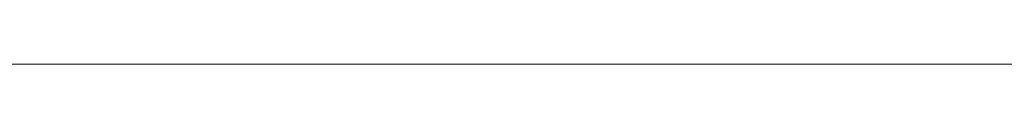
# Model space of a CAD drawing. Units: inches. Extents: x 459864 to 460310, y 324185 to 324787.
# Tile 94 of 112: x 460247.3904 to 460247.6764, y 324283.4832 to 324283.4832. Entities that reach past the tile are written whole.
import ezdxf

# ---------------------------------------------------------------- set-up
doc = ezdxf.new("R2010")
doc.units = ezdxf.units.IN
for name, color, linetype, lineweight in [('A-ANNO-DIMS', 2, 'Continuous', 18), ('L-HRDS', 9, 'Continuous', 18), ('L-SITE-PATT', 252, 'Continuous', 13)]:
    doc.layers.add(name, color=color, linetype=linetype, lineweight=lineweight)
doc.styles.get("Standard").update_dxf_attribs({"font": 'arial.ttf'})
doc.dimstyles.new('ISO-25', dxfattribs={"dimtxt": 6, "dimasz": 2.5, "dimexe": 1.25, "dimexo": 0.625, "dimtad": 1, "dimdec": 1, "dimlunit": 3, "dimtxsty": 'Standard', "dimcen": 2.5, "dimadec": 0, "dimazin": 0, "dimtfac": 1, "dimtdec": 1, "dimtmove": 0, "dimatfit": 3, "dimfxl": 1, "dimarcsym": 0})

# ---------------------------------------------------------------- blocks, each defined once
blk = doc.blocks.new('*D21')
at = {"layer": 'A-ANNO-DIMS', "color": 0, "lineweight": -2, "transparency": 16777216}
for p, q in [((460247.73993, 324715.48323), (460309.58037, 324715.48323)), ((460308.33037, 324712.98323), (460308.33037, 324285.98323)), ((460247.73993, 324283.48323), (460309.58037, 324283.48323))]:
    blk.add_line(p, q, dxfattribs=at)
at = {"layer": 'A-ANNO-DIMS', "color": 0, "transparency": 16777216}
for points in [[(460307.9137, 324712.98323), (460308.74704, 324712.98323), (460308.33037, 324715.48323)], [(460307.9137, 324285.98323), (460308.74704, 324285.98323), (460308.33037, 324283.48323)]]:
    blk.add_solid(points, dxfattribs=at)
at = {"layer": 'Defpoints', "color": 0, "transparency": 16777216}
for p in [(460247.11493, 324715.48323), (460247.11493, 324283.48323), (460308.33037, 324283.48323)]:
    blk.add_point(p, dxfattribs=at)
at = {"layer": 'A-ANNO-DIMS', "color": 0, "transparency": 16777216, "insert": (460304.63988, 324499.48323), "char_height": 6, "attachment_point": 5, "rotation": 90}
blk.add_mtext("36'", dxfattribs=at)

msp = doc.modelspace()

# ---------------------------------------------------------------- hatches: boundary and pattern name
at = {"layer": 'L-SITE-PATT'}
h = msp.add_hatch(dxfattribs=at)
h.set_pattern_fill('DOTS', color=256)
h.paths.add_polyline_path([(460269.80361, 324283.48323), (460247.11493, 324283.48323), (460121.92928, 324283.48323), (460121.92928, 324252.47302), (460117.42928, 324252.47302), (460110.12356, 324252.47302), (460110.12356, 324243.28654), (460080.82954, 324243.28654), (460080.82954, 324252.47302), (460061.11493, 324252.47302), (460061.11493, 324251.88242), (460077.9089, 324251.88242), (460077.9089, 324199.48323), (460080.82954, 324199.48323), (460080.82954, 324207.55322), (460110.12356, 324207.55322), (460110.12356, 324199.48323), (460110.81335, 324199.48323), (460262.11493, 324199.48323), (460269.80361, 324199.48323)], flags=17)
edge = h.paths.add_edge_path(flags=0)
edge.add_ellipse((460222.5903, 324263.81323), major_axis=(-8.48528, 8.48528), ratio=1, start_angle=405, end_angle=495, ccw=False)
edge.add_line((460214.82087, 324254.65989), (460214.83162, 324254.66592))
edge.add_ellipse((460222.5903, 324263.81323), major_axis=(-8.48528, 8.48528), ratio=1, start_angle=405, end_angle=495, ccw=False)
edge.add_line((460210.75891, 324261.78055), (460210.76758, 324261.78682))
edge.add_ellipse((460222.5903, 324263.81323), major_axis=(-8.48528, 8.48528), ratio=1, start_angle=405, end_angle=495, ccw=False)
edge.add_ellipse((460222.5903, 324263.81323), major_axis=(-8.48528, 8.48528), ratio=1, start_angle=392.754016, end_angle=405, ccw=False)
edge.add_ellipse((460222.5903, 324263.81323), major_axis=(-8.48528, 8.48528), ratio=1, start_angle=380.934718, end_angle=392.754016, ccw=False)
edge.add_line((460211.33706, 324267.98503), (460211.3404, 324267.98503))
edge.add_ellipse((460222.5903, 324263.81323), major_axis=(-8.48528, 8.48528), ratio=1, start_angle=380.934718, end_angle=392.754016, ccw=False)
edge.add_ellipse((460222.5903, 324263.81323), major_axis=(-8.48528, 8.48528), ratio=1, start_angle=347.901521, end_angle=380.934718, ccw=False)
edge.add_ellipse((460222.5903, 324263.81323), major_axis=(-8.48528, 8.48528), ratio=1, start_angle=327.061924, end_angle=347.901521, ccw=False)
edge.add_ellipse((460222.5903, 324263.81323), major_axis=(-8.48528, 8.48528), ratio=1, start_angle=278.324642, end_angle=327.061924, ccw=False)
edge.add_line((460225.15828, 324275.53599), (460225.1577, 324275.53464))
edge.add_ellipse((460222.5903, 324263.81323), major_axis=(-8.48528, 8.48528), ratio=1, start_angle=278.324642, end_angle=327.061924, ccw=False)
edge.add_ellipse((460222.5903, 324263.81323), major_axis=(-8.48528, 8.48528), ratio=1, start_angle=260.643569, end_angle=278.324642, ccw=False)
edge.add_ellipse((460222.5903, 324263.81323), major_axis=(-8.48528, 8.48528), ratio=1, start_angle=225, end_angle=260.643569, ccw=False)
edge.add_line((460234.50879, 324265.2428), (460234.50146, 324265.23944))
edge.add_ellipse((460222.5903, 324263.81323), major_axis=(-8.48528, 8.48528), ratio=1, start_angle=225, end_angle=260.643569, ccw=False)
edge.add_ellipse((460222.5903, 324263.81323), major_axis=(-8.48528, 8.48528), ratio=1, start_angle=495, end_angle=585, ccw=False)
edge.add_line((460234.43667, 324261.86121), (460234.42378, 324261.85782))
edge.add_ellipse((460222.5903, 324263.81323), major_axis=(-8.48528, 8.48528), ratio=1, start_angle=495, end_angle=585, ccw=False)
edge.add_line((460227.95013, 324253.06719), (460227.94641, 324253.08314))
edge.add_ellipse((460222.5903, 324263.81323), major_axis=(-8.48528, 8.48528), ratio=1, start_angle=495, end_angle=585, ccw=False)
edge.add_line((460226.22298, 324252.36927), (460226.21103, 324252.37955))
edge.add_ellipse((460222.5903, 324263.81323), major_axis=(-8.48528, 8.48528), ratio=1, start_angle=495, end_angle=585, ccw=False)
h.paths.add_polyline_path([(460219.65145, 324254.34665), (460218.46131, 324253.54498), (460218.27544, 324254.78932), (460219.6424, 324256.54177), (460219.62463, 324260.84756), (460216.11009, 324257.33302), (460214.34997, 324256.97807), (460215.41637, 324259.35568), (460212.52393, 324258.49582), (460213.13731, 324259.9298), (460218.50721, 324263.81323), (460222.5903, 324263.81323), (460222.5903, 324267.8067), (460218.17554, 324272.21231), (460219.02597, 324274.63898), (460222.5903, 324272.81113), (460222.5903, 324275.42332), (460223.0571, 324274.82493), (460222.67523, 324273.49221), (460225.91168, 324267.13461), (460219.62463, 324260.84756)], flags=0)
edge = h.paths.add_edge_path(flags=0)
edge.add_ellipse((460194.57576, 324264.04649), major_axis=(-8.48528, 8.48528), ratio=1, start_angle=495, end_angle=585, ccw=False)
edge.add_line((460199.93559, 324253.30046), (460199.93188, 324253.31641))
edge.add_ellipse((460194.57576, 324264.04649), major_axis=(-8.48528, 8.48528), ratio=1, start_angle=495, end_angle=585, ccw=False)
edge.add_line((460198.20844, 324252.60253), (460198.19649, 324252.61282))
edge.add_ellipse((460194.57576, 324264.04649), major_axis=(-8.48528, 8.48528), ratio=1, start_angle=495, end_angle=585, ccw=False)
edge.add_ellipse((460194.57576, 324264.04649), major_axis=(-8.48528, 8.48528), ratio=1, start_angle=405, end_angle=495, ccw=False)
edge.add_line((460186.80633, 324254.89316), (460186.81708, 324254.89919))
edge.add_ellipse((460194.57576, 324264.04649), major_axis=(-8.48528, 8.48528), ratio=1, start_angle=405, end_angle=495, ccw=False)
edge.add_line((460182.74437, 324262.01382), (460182.75305, 324262.02009))
edge.add_ellipse((460194.57576, 324264.04649), major_axis=(-8.48528, 8.48528), ratio=1, start_angle=405, end_angle=495, ccw=False)
edge.add_ellipse((460194.57576, 324264.04649), major_axis=(-8.48528, 8.48528), ratio=1, start_angle=392.754016, end_angle=405, ccw=False)
edge.add_ellipse((460194.57576, 324264.04649), major_axis=(-8.48528, 8.48528), ratio=1, start_angle=380.934718, end_angle=392.754016, ccw=False)
edge.add_line((460183.32252, 324268.21829), (460183.32587, 324268.21829))
edge.add_ellipse((460194.57576, 324264.04649), major_axis=(-8.48528, 8.48528), ratio=1, start_angle=380.934718, end_angle=392.754016, ccw=False)
edge.add_ellipse((460194.57576, 324264.04649), major_axis=(-8.48528, 8.48528), ratio=1, start_angle=347.901521, end_angle=380.934718, ccw=False)
edge.add_ellipse((460194.57576, 324264.04649), major_axis=(-8.48528, 8.48528), ratio=1, start_angle=327.061924, end_angle=347.901521, ccw=False)
edge.add_ellipse((460194.57576, 324264.04649), major_axis=(-8.48528, 8.48528), ratio=1, start_angle=278.324642, end_angle=327.061924, ccw=False)
edge.add_line((460197.14374, 324275.76926), (460197.14316, 324275.7679))
edge.add_ellipse((460194.57576, 324264.04649), major_axis=(-8.48528, 8.48528), ratio=1, start_angle=278.324642, end_angle=327.061924, ccw=False)
edge.add_ellipse((460194.57576, 324264.04649), major_axis=(-8.48528, 8.48528), ratio=1, start_angle=260.643569, end_angle=278.324642, ccw=False)
edge.add_ellipse((460194.57576, 324264.04649), major_axis=(-8.48528, 8.48528), ratio=1, start_angle=225, end_angle=260.643569, ccw=False)
edge.add_line((460206.49425, 324265.47606), (460206.48692, 324265.47271))
edge.add_ellipse((460194.57576, 324264.04649), major_axis=(-8.48528, 8.48528), ratio=1, start_angle=225, end_angle=260.643569, ccw=False)
edge.add_ellipse((460194.57576, 324264.04649), major_axis=(-8.48528, 8.48528), ratio=1, start_angle=495, end_angle=585, ccw=False)
edge.add_line((460206.42213, 324262.09448), (460206.40925, 324262.09109))
h.paths.add_polyline_path([(460191.61009, 324261.08083), (460191.63691, 324254.57992), (460190.44677, 324253.77825), (460190.2609, 324255.02259), (460191.62786, 324256.77503), (460191.61009, 324261.08083), (460188.09555, 324257.56629), (460186.33543, 324257.21133), (460187.40183, 324259.58894), (460184.5094, 324258.72909), (460185.12278, 324260.16306), (460190.49267, 324264.04649), (460194.57576, 324264.04649), (460194.57576, 324268.03996), (460190.161, 324272.44558), (460191.01143, 324274.87225), (460194.57576, 324273.04439), (460194.57576, 324275.65659), (460195.04256, 324275.0582), (460194.66069, 324273.72548), (460197.89714, 324267.36788)], flags=0)
edge = h.paths.add_edge_path(flags=0)
edge.add_ellipse((460252.91196, 324263.57762), major_axis=(-8.48528, 8.48528), ratio=1, start_angle=405, end_angle=495, ccw=False)
edge.add_line((460241.08058, 324261.54494), (460241.08925, 324261.55121))
edge.add_ellipse((460252.91196, 324263.57762), major_axis=(-8.48528, 8.48528), ratio=1, start_angle=405, end_angle=495, ccw=False)
edge.add_ellipse((460252.91196, 324263.57762), major_axis=(-8.48528, 8.48528), ratio=1, start_angle=392.754016, end_angle=405, ccw=False)
edge.add_ellipse((460252.91196, 324263.57762), major_axis=(-8.48528, 8.48528), ratio=1, start_angle=380.934718, end_angle=392.754016, ccw=False)
edge.add_line((460241.65872, 324267.74942), (460241.66207, 324267.74942))
edge.add_ellipse((460252.91196, 324263.57762), major_axis=(-8.48528, 8.48528), ratio=1, start_angle=380.934718, end_angle=392.754016, ccw=False)
edge.add_ellipse((460252.91196, 324263.57762), major_axis=(-8.48528, 8.48528), ratio=1, start_angle=347.901521, end_angle=380.934718, ccw=False)
edge.add_ellipse((460252.91196, 324263.57762), major_axis=(-8.48528, 8.48528), ratio=1, start_angle=327.061924, end_angle=347.901521, ccw=False)
edge.add_ellipse((460252.91196, 324263.57762), major_axis=(-8.48528, 8.48528), ratio=1, start_angle=278.324642, end_angle=327.061924, ccw=False)
edge.add_line((460255.47994, 324275.30038), (460255.47936, 324275.29902))
edge.add_ellipse((460252.91196, 324263.57762), major_axis=(-8.48528, 8.48528), ratio=1, start_angle=278.324642, end_angle=327.061924, ccw=False)
edge.add_ellipse((460252.91196, 324263.57762), major_axis=(-8.48528, 8.48528), ratio=1, start_angle=260.643569, end_angle=278.324642, ccw=False)
edge.add_ellipse((460252.91196, 324263.57762), major_axis=(-8.48528, 8.48528), ratio=1, start_angle=225, end_angle=260.643569, ccw=False)
edge.add_line((460264.83046, 324265.00718), (460264.82312, 324265.00383))
edge.add_ellipse((460252.91196, 324263.57762), major_axis=(-8.48528, 8.48528), ratio=1, start_angle=225, end_angle=260.643569, ccw=False)
edge.add_ellipse((460252.91196, 324263.57762), major_axis=(-8.48528, 8.48528), ratio=1, start_angle=495, end_angle=585, ccw=False)
edge.add_line((460264.75833, 324261.6256), (460264.74545, 324261.62221))
edge.add_ellipse((460252.91196, 324263.57762), major_axis=(-8.48528, 8.48528), ratio=1, start_angle=495, end_angle=585, ccw=False)
edge.add_line((460258.2718, 324252.83158), (460258.26808, 324252.84753))
edge.add_ellipse((460252.91196, 324263.57762), major_axis=(-8.48528, 8.48528), ratio=1, start_angle=495, end_angle=585, ccw=False)
edge.add_line((460256.54464, 324252.13365), (460256.5327, 324252.14394))
edge.add_ellipse((460252.91196, 324263.57762), major_axis=(-8.48528, 8.48528), ratio=1, start_angle=495, end_angle=585, ccw=False)
edge.add_ellipse((460252.91196, 324263.57762), major_axis=(-8.48528, 8.48528), ratio=1, start_angle=405, end_angle=495, ccw=False)
edge.add_line((460245.14253, 324254.42428), (460245.15329, 324254.43031))
h.paths.add_polyline_path([(460244.67163, 324256.74245), (460245.73803, 324259.12007), (460242.8456, 324258.26021), (460243.45898, 324259.69418), (460248.82888, 324263.57762), (460252.91196, 324263.57762), (460252.91196, 324267.57108), (460248.4972, 324271.9767), (460249.34763, 324274.40337), (460252.91196, 324272.57552), (460252.91196, 324275.18771), (460253.37876, 324274.58932), (460252.9969, 324273.2566), (460256.23334, 324266.899), (460249.9463, 324260.61195), (460249.97312, 324254.11104), (460248.78298, 324253.30937), (460248.5971, 324254.55371), (460249.96406, 324256.30615), (460249.9463, 324260.61195), (460246.43175, 324257.09741)], flags=0)
edge = h.paths.add_edge_path(flags=0)
edge.add_ellipse((460167.43869, 324262.83279), major_axis=(-8.48528, 8.48528), ratio=1, start_angle=495, end_angle=585, ccw=False)
edge.add_line((460172.79852, 324252.08676), (460172.79481, 324252.1027))
edge.add_ellipse((460167.43869, 324262.83279), major_axis=(-8.48528, 8.48528), ratio=1, start_angle=495, end_angle=585, ccw=False)
edge.add_line((460171.07137, 324251.38883), (460171.05942, 324251.39911))
edge.add_ellipse((460167.43869, 324262.83279), major_axis=(-8.48528, 8.48528), ratio=1, start_angle=495, end_angle=585, ccw=False)
edge.add_ellipse((460167.43869, 324262.83279), major_axis=(-8.48528, 8.48528), ratio=1, start_angle=405, end_angle=495, ccw=False)
edge.add_line((460159.66926, 324253.67945), (460159.68001, 324253.68548))
edge.add_ellipse((460167.43869, 324262.83279), major_axis=(-8.48528, 8.48528), ratio=1, start_angle=405, end_angle=495, ccw=False)
edge.add_line((460155.6073, 324260.80011), (460155.61598, 324260.80639))
edge.add_ellipse((460167.43869, 324262.83279), major_axis=(-8.48528, 8.48528), ratio=1, start_angle=405, end_angle=495, ccw=False)
edge.add_ellipse((460167.43869, 324262.83279), major_axis=(-8.48528, 8.48528), ratio=1, start_angle=392.754016, end_angle=405, ccw=False)
edge.add_ellipse((460167.43869, 324262.83279), major_axis=(-8.48528, 8.48528), ratio=1, start_angle=380.934718, end_angle=392.754016, ccw=False)
edge.add_line((460156.18545, 324267.00459), (460156.1888, 324267.00459))
edge.add_ellipse((460167.43869, 324262.83279), major_axis=(-8.48528, 8.48528), ratio=1, start_angle=380.934718, end_angle=392.754016, ccw=False)
edge.add_ellipse((460167.43869, 324262.83279), major_axis=(-8.48528, 8.48528), ratio=1, start_angle=347.901521, end_angle=380.934718, ccw=False)
edge.add_ellipse((460167.43869, 324262.83279), major_axis=(-8.48528, 8.48528), ratio=1, start_angle=327.061924, end_angle=347.901521, ccw=False)
edge.add_ellipse((460167.43869, 324262.83279), major_axis=(-8.48528, 8.48528), ratio=1, start_angle=278.324642, end_angle=327.061924, ccw=False)
edge.add_line((460170.00667, 324274.55555), (460170.00609, 324274.5542))
edge.add_ellipse((460167.43869, 324262.83279), major_axis=(-8.48528, 8.48528), ratio=1, start_angle=278.324642, end_angle=327.061924, ccw=False)
edge.add_ellipse((460167.43869, 324262.83279), major_axis=(-8.48528, 8.48528), ratio=1, start_angle=260.643569, end_angle=278.324642, ccw=False)
edge.add_ellipse((460167.43869, 324262.83279), major_axis=(-8.48528, 8.48528), ratio=1, start_angle=225, end_angle=260.643569, ccw=False)
edge.add_line((460179.35719, 324264.26236), (460179.34985, 324264.259))
edge.add_ellipse((460167.43869, 324262.83279), major_axis=(-8.48528, 8.48528), ratio=1, start_angle=225, end_angle=260.643569, ccw=False)
edge.add_ellipse((460167.43869, 324262.83279), major_axis=(-8.48528, 8.48528), ratio=1, start_angle=495, end_angle=585, ccw=False)
edge.add_line((460179.28506, 324260.88078), (460179.27218, 324260.87738))
h.paths.add_polyline_path([(460164.47302, 324259.86713), (460164.49985, 324253.36622), (460163.30971, 324252.56455), (460163.12383, 324253.80888), (460164.49079, 324255.56133), (460164.47302, 324259.86713), (460160.95848, 324256.35258), (460159.19836, 324255.99763), (460160.26476, 324258.37524), (460157.37233, 324257.51539), (460157.98571, 324258.94936), (460163.35561, 324262.83279), (460167.43869, 324262.83279), (460167.43869, 324266.82626), (460163.02393, 324271.23187), (460163.87436, 324273.65854), (460167.43869, 324271.83069), (460167.43869, 324274.44288), (460167.90549, 324273.84449), (460167.52362, 324272.51177), (460170.76007, 324266.15417)], flags=0)
edge = h.paths.add_edge_path(flags=0)
edge.add_ellipse((460140.75809, 324262.36958), major_axis=(-8.48528, 8.48528), ratio=1, start_angle=495, end_angle=585, ccw=False)
edge.add_line((460146.11792, 324251.62355), (460146.11421, 324251.6395))
edge.add_ellipse((460140.75809, 324262.36958), major_axis=(-8.48528, 8.48528), ratio=1, start_angle=495, end_angle=585, ccw=False)
edge.add_line((460144.39077, 324250.92562), (460144.37882, 324250.93591))
edge.add_ellipse((460140.75809, 324262.36958), major_axis=(-8.48528, 8.48528), ratio=1, start_angle=495, end_angle=585, ccw=False)
edge.add_ellipse((460140.75809, 324262.36958), major_axis=(-8.48528, 8.48528), ratio=1, start_angle=405, end_angle=495, ccw=False)
edge.add_line((460132.98866, 324253.21625), (460132.99941, 324253.22228))
edge.add_ellipse((460140.75809, 324262.36958), major_axis=(-8.48528, 8.48528), ratio=1, start_angle=405, end_angle=495, ccw=False)
edge.add_line((460128.9267, 324260.33691), (460128.93538, 324260.34318))
edge.add_ellipse((460140.75809, 324262.36958), major_axis=(-8.48528, 8.48528), ratio=1, start_angle=405, end_angle=495, ccw=False)
edge.add_ellipse((460140.75809, 324262.36958), major_axis=(-8.48528, 8.48528), ratio=1, start_angle=392.754016, end_angle=405, ccw=False)
edge.add_ellipse((460140.75809, 324262.36958), major_axis=(-8.48528, 8.48528), ratio=1, start_angle=380.934718, end_angle=392.754016, ccw=False)
edge.add_line((460129.50485, 324266.54138), (460129.5082, 324266.54138))
edge.add_ellipse((460140.75809, 324262.36958), major_axis=(-8.48528, 8.48528), ratio=1, start_angle=380.934718, end_angle=392.754016, ccw=False)
edge.add_ellipse((460140.75809, 324262.36958), major_axis=(-8.48528, 8.48528), ratio=1, start_angle=347.901521, end_angle=380.934718, ccw=False)
edge.add_ellipse((460140.75809, 324262.36958), major_axis=(-8.48528, 8.48528), ratio=1, start_angle=327.061924, end_angle=347.901521, ccw=False)
edge.add_ellipse((460140.75809, 324262.36958), major_axis=(-8.48528, 8.48528), ratio=1, start_angle=278.324642, end_angle=327.061924, ccw=False)
edge.add_line((460143.32607, 324274.09235), (460143.32549, 324274.09099))
edge.add_ellipse((460140.75809, 324262.36958), major_axis=(-8.48528, 8.48528), ratio=1, start_angle=278.324642, end_angle=327.061924, ccw=False)
edge.add_ellipse((460140.75809, 324262.36958), major_axis=(-8.48528, 8.48528), ratio=1, start_angle=260.643569, end_angle=278.324642, ccw=False)
edge.add_ellipse((460140.75809, 324262.36958), major_axis=(-8.48528, 8.48528), ratio=1, start_angle=225, end_angle=260.643569, ccw=False)
edge.add_line((460152.67658, 324263.79915), (460152.66925, 324263.7958))
edge.add_ellipse((460140.75809, 324262.36958), major_axis=(-8.48528, 8.48528), ratio=1, start_angle=225, end_angle=260.643569, ccw=False)
edge.add_ellipse((460140.75809, 324262.36958), major_axis=(-8.48528, 8.48528), ratio=1, start_angle=495, end_angle=585, ccw=False)
edge.add_line((460152.60446, 324260.41757), (460152.59158, 324260.41418))
h.paths.add_polyline_path([(460137.79242, 324259.40392), (460137.81925, 324252.90301), (460136.6291, 324252.10134), (460136.44323, 324253.34568), (460137.81019, 324255.09812), (460137.79242, 324259.40392), (460134.27788, 324255.88938), (460132.51776, 324255.53442), (460133.58416, 324257.91203), (460130.69173, 324257.05218), (460131.30511, 324258.48615), (460136.675, 324262.36958), (460140.75809, 324262.36958), (460140.75809, 324266.36305), (460136.34333, 324270.76867), (460137.19376, 324273.19534), (460140.75809, 324271.36749), (460140.75809, 324273.97968), (460141.22489, 324273.38129), (460140.84302, 324272.04857), (460144.07947, 324265.69097)], flags=0)
h.paths.add_polyline_path([(460110.12356, 324227.41387), (460080.82954, 324227.41387), (460080.82954, 324235.48385), (460110.12356, 324235.48385)], flags=16)
h.paths.add_polyline_path([(460110.12356, 324220.79663), (460110.12356, 324212.72665), (460080.82954, 324212.72665), (460080.82954, 324220.79663)], flags=16)
h.paths.add_polyline_path([(460269.80361, 324283.48323), (460247.11493, 324283.48323), (460121.92928, 324283.48323), (460121.92928, 324252.47302), (460117.42928, 324252.47302), (460110.12356, 324252.47302), (460110.12356, 324243.28654), (460080.82954, 324243.28654), (460080.82954, 324252.47302), (460061.11493, 324252.47302), (460061.11493, 324251.88242), (460077.9089, 324251.88242), (460077.9089, 324199.48323), (460080.82954, 324199.48323), (460080.82954, 324207.55322), (460110.12356, 324207.55322), (460110.12356, 324199.48323), (460262.11493, 324199.48323), (460269.80361, 324199.48323)], flags=17)
h.paths.add_polyline_path([(460219.65145, 324254.34665), (460218.46131, 324253.54498), (460218.27544, 324254.78932), (460219.6424, 324256.54177), (460219.62463, 324260.84756), (460216.11009, 324257.33302), (460214.34997, 324256.97807), (460215.41637, 324259.35568), (460212.52393, 324258.49582), (460213.13731, 324259.9298), (460218.50721, 324263.81323), (460222.5903, 324263.81323), (460220.18049, 324266.22304), (460215.46096, 324265.30765), (460211.83453, 324266.13655), (460216.24662, 324267.98503), (460218.4185, 324267.98503), (460222.5903, 324263.81323), (460222.5903, 324267.8067), (460218.17554, 324272.21231), (460219.02597, 324274.63898), (460222.5903, 324272.81113), (460222.5903, 324275.42332), (460223.0571, 324274.82493), (460222.67523, 324273.49221), (460225.91168, 324267.13461), (460222.5903, 324263.81323), (460231.38287, 324263.81323), (460228.48472, 324262.48783), (460224.42521, 324261.97832), (460228.6799, 324257.72362), (460228.96584, 324254.79101), (460227.14177, 324256.53663), (460227.54207, 324254.81857), (460227.33334, 324253.61447), (460222.5903, 324259.98463), (460222.5903, 324255.49667), (460221.37741, 324256.54085), (460220.57579, 324261.79873), (460219.62463, 324260.84756)], flags=0)
h.paths.add_polyline_path([(460199.12723, 324256.7699), (460199.52753, 324255.05184), (460199.31881, 324253.84773), (460194.57576, 324260.21789), (460194.57576, 324255.72993), (460193.36287, 324256.77411), (460192.56126, 324262.03199), (460191.61009, 324261.08083), (460191.63691, 324254.57992), (460190.44677, 324253.77825), (460190.2609, 324255.02259), (460191.62786, 324256.77503), (460191.61009, 324261.08083), (460188.09555, 324257.56629), (460186.33543, 324257.21133), (460187.40183, 324259.58894), (460184.5094, 324258.72909), (460185.12278, 324260.16306), (460190.49267, 324264.04649), (460194.57576, 324264.04649), (460192.16595, 324266.4563), (460187.44642, 324265.54091), (460183.82, 324266.36982), (460188.23208, 324268.21829), (460190.40396, 324268.21829), (460194.57576, 324264.04649), (460194.57576, 324268.03996), (460190.161, 324272.44558), (460191.01143, 324274.87225), (460194.57576, 324273.04439), (460194.57576, 324275.65659), (460195.04256, 324275.0582), (460194.66069, 324273.72548), (460197.89714, 324267.36788), (460194.57576, 324264.04649), (460203.36833, 324264.04649), (460200.47018, 324262.72109), (460196.41067, 324262.21158), (460200.66536, 324257.95689), (460200.9513, 324255.02428)], flags=0)
h.paths.add_polyline_path([(460244.67163, 324256.74245), (460245.73803, 324259.12007), (460242.8456, 324258.26021), (460243.45898, 324259.69418), (460248.82888, 324263.57762), (460252.91196, 324263.57762), (460250.50215, 324265.98742), (460245.78262, 324265.07203), (460242.1562, 324265.90094), (460246.56828, 324267.74942), (460248.74016, 324267.74942), (460252.91196, 324263.57762), (460252.91196, 324267.57108), (460248.4972, 324271.9767), (460249.34763, 324274.40337), (460252.91196, 324272.57552), (460252.91196, 324275.18771), (460253.37876, 324274.58932), (460252.9969, 324273.2566), (460256.23334, 324266.899), (460252.91196, 324263.57762), (460261.70454, 324263.57762), (460258.80638, 324262.25221), (460254.74687, 324261.7427), (460259.00157, 324257.48801), (460259.2875, 324254.5554), (460257.46343, 324256.30102), (460257.86373, 324254.58296), (460257.65501, 324253.37885), (460252.91196, 324259.74901), (460252.91196, 324255.26105), (460251.69907, 324256.30524), (460250.89746, 324261.56311), (460249.9463, 324260.61195), (460249.97312, 324254.11104), (460248.78298, 324253.30937), (460248.5971, 324254.55371), (460249.96406, 324256.30615), (460249.9463, 324260.61195), (460246.43175, 324257.09741)], flags=0)
h.paths.add_polyline_path([(460173.52829, 324256.74319), (460173.81423, 324253.81058), (460171.99016, 324255.55619), (460172.39046, 324253.83814), (460172.18174, 324252.63403), (460167.43869, 324259.00419), (460167.43869, 324254.51623), (460166.2258, 324255.56041), (460165.42419, 324260.81829), (460164.47302, 324259.86713), (460164.49985, 324253.36622), (460163.30971, 324252.56455), (460163.12383, 324253.80888), (460164.49079, 324255.56133), (460164.47302, 324259.86713), (460160.95848, 324256.35258), (460159.19836, 324255.99763), (460160.26476, 324258.37524), (460157.37233, 324257.51539), (460157.98571, 324258.94936), (460163.35561, 324262.83279), (460167.43869, 324262.83279), (460165.02888, 324265.2426), (460160.30935, 324264.32721), (460156.68293, 324265.15611), (460161.09501, 324267.00459), (460163.26689, 324267.00459), (460167.43869, 324262.83279), (460167.43869, 324266.82626), (460163.02393, 324271.23187), (460163.87436, 324273.65854), (460167.43869, 324271.83069), (460167.43869, 324274.44288), (460167.90549, 324273.84449), (460167.52362, 324272.51177), (460170.76007, 324266.15417), (460167.43869, 324262.83279), (460176.23127, 324262.83279), (460173.33311, 324261.50739), (460169.2736, 324260.99788)], flags=0)
h.paths.add_polyline_path([(460146.84769, 324256.27998), (460147.13363, 324253.34737), (460145.30956, 324255.09299), (460145.70986, 324253.37493), (460145.50114, 324252.17082), (460140.75809, 324258.54098), (460140.75809, 324254.05302), (460139.5452, 324255.0972), (460138.74359, 324260.35508), (460137.79242, 324259.40392), (460137.81925, 324252.90301), (460136.6291, 324252.10134), (460136.44323, 324253.34568), (460137.81019, 324255.09812), (460137.79242, 324259.40392), (460134.27788, 324255.88938), (460132.51776, 324255.53442), (460133.58416, 324257.91203), (460130.69173, 324257.05218), (460131.30511, 324258.48615), (460136.675, 324262.36958), (460140.75809, 324262.36958), (460138.34828, 324264.77939), (460133.62875, 324263.864), (460130.00233, 324264.69291), (460134.41441, 324266.54138), (460136.58629, 324266.54138), (460140.75809, 324262.36958), (460140.75809, 324266.36305), (460136.34333, 324270.76867), (460137.19376, 324273.19534), (460140.75809, 324271.36749), (460140.75809, 324273.97968), (460141.22489, 324273.38129), (460140.84302, 324272.04857), (460144.07947, 324265.69097), (460140.75809, 324262.36958), (460149.55066, 324262.36958), (460146.65251, 324261.04418), (460142.593, 324260.53467)], flags=0)
edge = h.paths.add_edge_path()
edge.add_line((460269.80361, 324272.54905), (460260.88148, 324272.54905))
edge.add_ellipse((460252.91196, 324263.57762), major_axis=(-8.48528, 8.48528), ratio=1, start_angle=260.643569, end_angle=273.384624, ccw=False)
edge.add_line((460262.28261, 324271.09211), (460262.26055, 324271.09106))
edge.add_ellipse((460252.91196, 324263.57762), major_axis=(-8.48528, 8.48528), ratio=1, start_angle=260.643569, end_angle=273.384624, ccw=False)
edge.add_ellipse((460252.91196, 324263.57762), major_axis=(-8.48528, 8.48528), ratio=1, start_angle=225, end_angle=260.643569, ccw=False)
edge.add_line((460263.60857, 324269.06329), (460263.57165, 324269.05828))
edge.add_ellipse((460252.91196, 324263.57762), major_axis=(-8.48528, 8.48528), ratio=1, start_angle=225, end_angle=260.643569, ccw=False)
edge.add_line((460264.61546, 324266.30554), (460264.58536, 324266.3052))
edge.add_ellipse((460252.91196, 324263.57762), major_axis=(-8.48528, 8.48528), ratio=1, start_angle=225, end_angle=260.643569, ccw=False)
edge.add_line((460264.83046, 324265.00718), (460264.82312, 324265.00383))
edge.add_ellipse((460252.91196, 324263.57762), major_axis=(-8.48528, 8.48528), ratio=1, start_angle=225, end_angle=260.643569, ccw=False)
edge.add_ellipse((460252.91196, 324263.57762), major_axis=(-8.48528, 8.48528), ratio=1, start_angle=495, end_angle=585, ccw=False)
edge.add_line((460264.75833, 324261.6256), (460264.74545, 324261.62221))
edge.add_ellipse((460252.91196, 324263.57762), major_axis=(-8.48528, 8.48528), ratio=1, start_angle=495, end_angle=585, ccw=False)
edge.add_line((460263.4422, 324257.73902), (460263.38926, 324257.77924))
edge.add_ellipse((460252.91196, 324263.57762), major_axis=(-8.48528, 8.48528), ratio=1, start_angle=495, end_angle=585, ccw=False)
edge.add_line((460258.12807, 324252.7435), (460258.10188, 324252.77868))
edge.add_ellipse((460252.91196, 324263.57762), major_axis=(-8.48528, 8.48528), ratio=1, start_angle=495, end_angle=585, ccw=False)
edge.add_line((460256.54464, 324252.13365), (460256.5327, 324252.14394))
edge.add_ellipse((460252.91196, 324263.57762), major_axis=(-8.48528, 8.48528), ratio=1, start_angle=495, end_angle=585, ccw=False)
edge.add_ellipse((460252.91196, 324263.57762), major_axis=(-8.48528, 8.48528), ratio=1, start_angle=405, end_angle=495, ccw=False)
edge.add_line((460250.59399, 324251.78041), (460250.60465, 324251.81982))
edge.add_ellipse((460252.91196, 324263.57762), major_axis=(-8.48528, 8.48528), ratio=1, start_angle=405, end_angle=495, ccw=False)
edge.add_line((460245.14253, 324254.42428), (460245.15329, 324254.43031))
edge.add_ellipse((460252.91196, 324263.57762), major_axis=(-8.48528, 8.48528), ratio=1, start_angle=405, end_angle=495, ccw=False)
edge.add_line((460243.52459, 324256.059), (460243.56034, 324256.09136))
edge.add_ellipse((460252.91196, 324263.57762), major_axis=(-8.48528, 8.48528), ratio=1, start_angle=405, end_angle=495, ccw=False)
edge.add_line((460241.4401, 324259.89273), (460241.52244, 324259.89588))
edge.add_ellipse((460252.91196, 324263.57762), major_axis=(-8.48528, 8.48528), ratio=1, start_angle=405, end_angle=495, ccw=False)
edge.add_line((460241.08058, 324261.54494), (460241.08925, 324261.55121))
edge.add_ellipse((460252.91196, 324263.57762), major_axis=(-8.48528, 8.48528), ratio=1, start_angle=405, end_angle=495, ccw=False)
edge.add_ellipse((460252.91196, 324263.57762), major_axis=(-8.48528, 8.48528), ratio=1, start_angle=392.754016, end_angle=405, ccw=False)
edge.add_line((460241.0503, 324265.43761), (460241.06257, 324265.44275))
edge.add_ellipse((460252.91196, 324263.57762), major_axis=(-8.48528, 8.48528), ratio=1, start_angle=392.754016, end_angle=405, ccw=False)
edge.add_ellipse((460252.91196, 324263.57762), major_axis=(-8.48528, 8.48528), ratio=1, start_angle=380.934718, end_angle=392.754016, ccw=False)
edge.add_line((460241.45189, 324267.17639), (460241.46904, 324267.17099))
edge.add_ellipse((460252.91196, 324263.57762), major_axis=(-8.48528, 8.48528), ratio=1, start_angle=380.934718, end_angle=392.754016, ccw=False)
edge.add_line((460241.65872, 324267.74942), (460241.66207, 324267.74942))
edge.add_ellipse((460252.91196, 324263.57762), major_axis=(-8.48528, 8.48528), ratio=1, start_angle=380.934718, end_angle=392.754016, ccw=False)
edge.add_ellipse((460252.91196, 324263.57762), major_axis=(-8.48528, 8.48528), ratio=1, start_angle=356.615376, end_angle=380.934718, ccw=False)
edge.add_line((460244.88029, 324272.48765), (460244.71265, 324272.54905))
edge.add_line((460244.71265, 324272.54905), (460230.81741, 324272.54905))
edge.add_ellipse((460222.5903, 324263.81323), major_axis=(-8.48528, 8.48528), ratio=1, start_angle=260.643569, end_angle=271.717775, ccw=False)
edge.add_ellipse((460222.5903, 324263.81323), major_axis=(-8.48528, 8.48528), ratio=1, start_angle=225, end_angle=260.643569, ccw=False)
edge.add_line((460233.2869, 324269.29891), (460233.24999, 324269.2939))
edge.add_ellipse((460222.5903, 324263.81323), major_axis=(-8.48528, 8.48528), ratio=1, start_angle=225, end_angle=260.643569, ccw=False)
edge.add_line((460234.2938, 324266.54115), (460234.26369, 324266.54081))
edge.add_ellipse((460222.5903, 324263.81323), major_axis=(-8.48528, 8.48528), ratio=1, start_angle=225, end_angle=260.643569, ccw=False)
edge.add_line((460234.50879, 324265.2428), (460234.50146, 324265.23944))
edge.add_ellipse((460222.5903, 324263.81323), major_axis=(-8.48528, 8.48528), ratio=1, start_angle=225, end_angle=260.643569, ccw=False)
edge.add_ellipse((460222.5903, 324263.81323), major_axis=(-8.48528, 8.48528), ratio=1, start_angle=495, end_angle=585, ccw=False)
edge.add_line((460234.43667, 324261.86121), (460234.42378, 324261.85782))
edge.add_ellipse((460222.5903, 324263.81323), major_axis=(-8.48528, 8.48528), ratio=1, start_angle=495, end_angle=585, ccw=False)
edge.add_line((460233.12054, 324257.97463), (460233.06759, 324258.01485))
edge.add_ellipse((460222.5903, 324263.81323), major_axis=(-8.48528, 8.48528), ratio=1, start_angle=495, end_angle=585, ccw=False)
edge.add_line((460227.8064, 324252.97912), (460227.78021, 324253.0143))
edge.add_ellipse((460222.5903, 324263.81323), major_axis=(-8.48528, 8.48528), ratio=1, start_angle=495, end_angle=585, ccw=False)
edge.add_line((460226.22298, 324252.36927), (460226.21103, 324252.37955))
edge.add_ellipse((460222.5903, 324263.81323), major_axis=(-8.48528, 8.48528), ratio=1, start_angle=495, end_angle=585, ccw=False)
edge.add_ellipse((460222.5903, 324263.81323), major_axis=(-8.48528, 8.48528), ratio=1, start_angle=405, end_angle=495, ccw=False)
edge.add_line((460220.27232, 324252.01602), (460220.28299, 324252.05543))
edge.add_ellipse((460222.5903, 324263.81323), major_axis=(-8.48528, 8.48528), ratio=1, start_angle=405, end_angle=495, ccw=False)
edge.add_line((460214.82087, 324254.65989), (460214.83162, 324254.66592))
edge.add_ellipse((460222.5903, 324263.81323), major_axis=(-8.48528, 8.48528), ratio=1, start_angle=405, end_angle=495, ccw=False)
edge.add_line((460213.20292, 324256.29462), (460213.23868, 324256.32697))
edge.add_ellipse((460222.5903, 324263.81323), major_axis=(-8.48528, 8.48528), ratio=1, start_angle=405, end_angle=495, ccw=False)
edge.add_line((460211.11844, 324260.12834), (460211.20077, 324260.13149))
edge.add_ellipse((460222.5903, 324263.81323), major_axis=(-8.48528, 8.48528), ratio=1, start_angle=405, end_angle=495, ccw=False)
edge.add_line((460210.75891, 324261.78055), (460210.76758, 324261.78682))
edge.add_ellipse((460222.5903, 324263.81323), major_axis=(-8.48528, 8.48528), ratio=1, start_angle=405, end_angle=495, ccw=False)
edge.add_ellipse((460222.5903, 324263.81323), major_axis=(-8.48528, 8.48528), ratio=1, start_angle=392.754016, end_angle=405, ccw=False)
edge.add_line((460210.72863, 324265.67323), (460210.7409, 324265.67836))
edge.add_ellipse((460222.5903, 324263.81323), major_axis=(-8.48528, 8.48528), ratio=1, start_angle=392.754016, end_angle=405, ccw=False)
edge.add_ellipse((460222.5903, 324263.81323), major_axis=(-8.48528, 8.48528), ratio=1, start_angle=380.934718, end_angle=392.754016, ccw=False)
edge.add_line((460211.13022, 324267.412), (460211.14738, 324267.4066))
edge.add_ellipse((460222.5903, 324263.81323), major_axis=(-8.48528, 8.48528), ratio=1, start_angle=380.934718, end_angle=392.754016, ccw=False)
edge.add_line((460211.33706, 324267.98503), (460211.3404, 324267.98503))
edge.add_ellipse((460222.5903, 324263.81323), major_axis=(-8.48528, 8.48528), ratio=1, start_angle=380.934718, end_angle=392.754016, ccw=False)
edge.add_ellipse((460222.5903, 324263.81323), major_axis=(-8.48528, 8.48528), ratio=1, start_angle=358.282225, end_angle=380.934718, ccw=False)
edge.add_line((460213.70452, 324271.90183), (460213.70904, 324271.86897))
edge.add_ellipse((460222.5903, 324263.81323), major_axis=(-8.48528, 8.48528), ratio=1, start_angle=358.282225, end_angle=380.934718, ccw=False)
edge.add_line((460214.36318, 324272.54905), (460203.07832, 324272.54905))
edge.add_line((460203.07832, 324272.54905), (460203.06034, 324272.53108))
edge.add_ellipse((460194.57576, 324264.04649), major_axis=(-8.48528, 8.48528), ratio=1, start_angle=260.643569, end_angle=270.11679, ccw=False)
edge.add_line((460203.95659, 324271.56147), (460203.92091, 324271.55978))
edge.add_ellipse((460194.57576, 324264.04649), major_axis=(-8.48528, 8.48528), ratio=1, start_angle=260.643569, end_angle=270.11679, ccw=False)
edge.add_ellipse((460194.57576, 324264.04649), major_axis=(-8.48528, 8.48528), ratio=1, start_angle=225, end_angle=260.643569, ccw=False)
edge.add_line((460205.27237, 324269.53217), (460205.23545, 324269.52716))
edge.add_ellipse((460194.57576, 324264.04649), major_axis=(-8.48528, 8.48528), ratio=1, start_angle=225, end_angle=260.643569, ccw=False)
edge.add_line((460206.27926, 324266.77442), (460206.24915, 324266.77407))
edge.add_ellipse((460194.57576, 324264.04649), major_axis=(-8.48528, 8.48528), ratio=1, start_angle=225, end_angle=260.643569, ccw=False)
edge.add_line((460206.49425, 324265.47606), (460206.48692, 324265.47271))
edge.add_ellipse((460194.57576, 324264.04649), major_axis=(-8.48528, 8.48528), ratio=1, start_angle=225, end_angle=260.643569, ccw=False)
edge.add_ellipse((460194.57576, 324264.04649), major_axis=(-8.48528, 8.48528), ratio=1, start_angle=495, end_angle=585, ccw=False)
edge.add_line((460206.42213, 324262.09448), (460206.40925, 324262.09109))
edge.add_ellipse((460194.57576, 324264.04649), major_axis=(-8.48528, 8.48528), ratio=1, start_angle=495, end_angle=585, ccw=False)
edge.add_line((460205.106, 324258.2079), (460205.05306, 324258.24812))
edge.add_ellipse((460194.57576, 324264.04649), major_axis=(-8.48528, 8.48528), ratio=1, start_angle=495, end_angle=585, ccw=False)
edge.add_line((460199.79187, 324253.21238), (460199.76568, 324253.24756))
edge.add_ellipse((460194.57576, 324264.04649), major_axis=(-8.48528, 8.48528), ratio=1, start_angle=495, end_angle=585, ccw=False)
edge.add_line((460198.20844, 324252.60253), (460198.19649, 324252.61282))
edge.add_ellipse((460194.57576, 324264.04649), major_axis=(-8.48528, 8.48528), ratio=1, start_angle=495, end_angle=585, ccw=False)
edge.add_ellipse((460194.57576, 324264.04649), major_axis=(-8.48528, 8.48528), ratio=1, start_angle=405, end_angle=495, ccw=False)
edge.add_line((460192.25779, 324252.24929), (460192.26845, 324252.2887))
edge.add_ellipse((460194.57576, 324264.04649), major_axis=(-8.48528, 8.48528), ratio=1, start_angle=405, end_angle=495, ccw=False)
edge.add_line((460186.80633, 324254.89316), (460186.81708, 324254.89919))
edge.add_ellipse((460194.57576, 324264.04649), major_axis=(-8.48528, 8.48528), ratio=1, start_angle=405, end_angle=495, ccw=False)
edge.add_line((460185.18839, 324256.52788), (460185.22414, 324256.56024))
edge.add_ellipse((460194.57576, 324264.04649), major_axis=(-8.48528, 8.48528), ratio=1, start_angle=405, end_angle=495, ccw=False)
edge.add_line((460183.1039, 324260.3616), (460183.18624, 324260.36476))
edge.add_ellipse((460194.57576, 324264.04649), major_axis=(-8.48528, 8.48528), ratio=1, start_angle=405, end_angle=495, ccw=False)
edge.add_line((460182.74437, 324262.01382), (460182.75305, 324262.02009))
edge.add_ellipse((460194.57576, 324264.04649), major_axis=(-8.48528, 8.48528), ratio=1, start_angle=405, end_angle=495, ccw=False)
edge.add_ellipse((460194.57576, 324264.04649), major_axis=(-8.48528, 8.48528), ratio=1, start_angle=392.754016, end_angle=405, ccw=False)
edge.add_line((460182.7141, 324265.90649), (460182.72636, 324265.91163))
edge.add_ellipse((460194.57576, 324264.04649), major_axis=(-8.48528, 8.48528), ratio=1, start_angle=392.754016, end_angle=405, ccw=False)
edge.add_ellipse((460194.57576, 324264.04649), major_axis=(-8.48528, 8.48528), ratio=1, start_angle=380.934718, end_angle=392.754016, ccw=False)
edge.add_line((460183.11568, 324267.64527), (460183.13284, 324267.63987))
edge.add_ellipse((460194.57576, 324264.04649), major_axis=(-8.48528, 8.48528), ratio=1, start_angle=380.934718, end_angle=392.754016, ccw=False)
edge.add_line((460183.32252, 324268.21829), (460183.32587, 324268.21829))
edge.add_ellipse((460194.57576, 324264.04649), major_axis=(-8.48528, 8.48528), ratio=1, start_angle=380.934718, end_angle=392.754016, ccw=False)
edge.add_ellipse((460194.57576, 324264.04649), major_axis=(-8.48528, 8.48528), ratio=1, start_angle=359.88321, end_angle=380.934718, ccw=False)
edge.add_line((460184.49136, 324270.61077), (460184.55315, 324270.61077))
edge.add_ellipse((460194.57576, 324264.04649), major_axis=(-8.48528, 8.48528), ratio=1, start_angle=359.88321, end_angle=380.934718, ccw=False)
edge.add_line((460185.34584, 324271.76024), (460185.37863, 324271.72802))
edge.add_ellipse((460194.57576, 324264.04649), major_axis=(-8.48528, 8.48528), ratio=1, start_angle=359.88321, end_angle=380.934718, ccw=False)
edge.add_line((460185.69672, 324272.08618), (460185.633, 324272.54905))
edge.add_line((460185.633, 324272.54905), (460174.68345, 324272.54905))
edge.add_line((460174.68345, 324272.54905), (460174.60605, 324272.45718))
edge.add_ellipse((460167.43869, 324262.83279), major_axis=(-8.48528, 8.48528), ratio=1, start_angle=260.643569, end_angle=278.324642, ccw=False)
edge.add_ellipse((460167.43869, 324262.83279), major_axis=(-8.48528, 8.48528), ratio=1, start_angle=225, end_angle=260.643569, ccw=False)
edge.add_line((460178.1353, 324268.31847), (460178.09838, 324268.31346))
edge.add_ellipse((460167.43869, 324262.83279), major_axis=(-8.48528, 8.48528), ratio=1, start_angle=225, end_angle=260.643569, ccw=False)
edge.add_line((460179.14219, 324265.56072), (460179.11209, 324265.56037))
edge.add_ellipse((460167.43869, 324262.83279), major_axis=(-8.48528, 8.48528), ratio=1, start_angle=225, end_angle=260.643569, ccw=False)
edge.add_line((460179.35719, 324264.26236), (460179.34985, 324264.259))
edge.add_ellipse((460167.43869, 324262.83279), major_axis=(-8.48528, 8.48528), ratio=1, start_angle=225, end_angle=260.643569, ccw=False)
edge.add_ellipse((460167.43869, 324262.83279), major_axis=(-8.48528, 8.48528), ratio=1, start_angle=495, end_angle=585, ccw=False)
edge.add_line((460179.28506, 324260.88078), (460179.27218, 324260.87738))
edge.add_ellipse((460167.43869, 324262.83279), major_axis=(-8.48528, 8.48528), ratio=1, start_angle=495, end_angle=585, ccw=False)
edge.add_line((460177.96893, 324256.99419), (460177.91599, 324257.03442))
edge.add_ellipse((460167.43869, 324262.83279), major_axis=(-8.48528, 8.48528), ratio=1, start_angle=495, end_angle=585, ccw=False)
edge.add_line((460172.6548, 324251.99868), (460172.62861, 324252.03386))
edge.add_ellipse((460167.43869, 324262.83279), major_axis=(-8.48528, 8.48528), ratio=1, start_angle=495, end_angle=585, ccw=False)
edge.add_line((460171.07137, 324251.38883), (460171.05942, 324251.39911))
edge.add_ellipse((460167.43869, 324262.83279), major_axis=(-8.48528, 8.48528), ratio=1, start_angle=495, end_angle=585, ccw=False)
edge.add_ellipse((460167.43869, 324262.83279), major_axis=(-8.48528, 8.48528), ratio=1, start_angle=405, end_angle=495, ccw=False)
edge.add_line((460165.12072, 324251.03559), (460165.13138, 324251.07499))
edge.add_ellipse((460167.43869, 324262.83279), major_axis=(-8.48528, 8.48528), ratio=1, start_angle=405, end_angle=495, ccw=False)
edge.add_line((460159.66926, 324253.67945), (460159.68001, 324253.68548))
edge.add_ellipse((460167.43869, 324262.83279), major_axis=(-8.48528, 8.48528), ratio=1, start_angle=405, end_angle=495, ccw=False)
edge.add_line((460158.05132, 324255.31418), (460158.08707, 324255.34654))
edge.add_ellipse((460167.43869, 324262.83279), major_axis=(-8.48528, 8.48528), ratio=1, start_angle=405, end_angle=495, ccw=False)
edge.add_line((460155.96683, 324259.1479), (460156.04917, 324259.15105))
edge.add_ellipse((460167.43869, 324262.83279), major_axis=(-8.48528, 8.48528), ratio=1, start_angle=405, end_angle=495, ccw=False)
edge.add_line((460155.6073, 324260.80011), (460155.61598, 324260.80639))
edge.add_ellipse((460167.43869, 324262.83279), major_axis=(-8.48528, 8.48528), ratio=1, start_angle=405, end_angle=495, ccw=False)
edge.add_ellipse((460167.43869, 324262.83279), major_axis=(-8.48528, 8.48528), ratio=1, start_angle=392.754016, end_angle=405, ccw=False)
edge.add_line((460155.57703, 324264.69279), (460155.58929, 324264.69793))
edge.add_ellipse((460167.43869, 324262.83279), major_axis=(-8.48528, 8.48528), ratio=1, start_angle=392.754016, end_angle=405, ccw=False)
edge.add_ellipse((460167.43869, 324262.83279), major_axis=(-8.48528, 8.48528), ratio=1, start_angle=380.934718, end_angle=392.754016, ccw=False)
edge.add_line((460155.97862, 324266.43157), (460155.99577, 324266.42616))
edge.add_ellipse((460167.43869, 324262.83279), major_axis=(-8.48528, 8.48528), ratio=1, start_angle=380.934718, end_angle=392.754016, ccw=False)
edge.add_line((460156.18545, 324267.00459), (460156.1888, 324267.00459))
edge.add_ellipse((460167.43869, 324262.83279), major_axis=(-8.48528, 8.48528), ratio=1, start_angle=380.934718, end_angle=392.754016, ccw=False)
edge.add_ellipse((460167.43869, 324262.83279), major_axis=(-8.48528, 8.48528), ratio=1, start_angle=350.934486, end_angle=380.934718, ccw=False)
edge.add_line((460157.36328, 324269.39707), (460157.41439, 324269.39707))
edge.add_ellipse((460167.43869, 324262.83279), major_axis=(-8.48528, 8.48528), ratio=1, start_angle=350.934486, end_angle=380.934718, ccw=False)
edge.add_line((460158.22053, 324270.53498), (460158.23648, 324270.51931))
edge.add_ellipse((460167.43869, 324262.83279), major_axis=(-8.48528, 8.48528), ratio=1, start_angle=350.934486, end_angle=380.934718, ccw=False)
edge.add_line((460159.37944, 324271.75293), (460159.41931, 324271.73833))
edge.add_ellipse((460167.43869, 324262.83279), major_axis=(-8.48528, 8.48528), ratio=1, start_angle=350.934486, end_angle=380.934718, ccw=False)
edge.add_line((460160.39637, 324272.54905), (460147.11249, 324272.54905))
edge.add_ellipse((460140.75809, 324262.36958), major_axis=(-8.48528, 8.48528), ratio=1, start_angle=278.324642, end_angle=283.026071, ccw=False)
edge.add_ellipse((460140.75809, 324262.36958), major_axis=(-8.48528, 8.48528), ratio=1, start_angle=260.643569, end_angle=278.324642, ccw=False)
edge.add_ellipse((460140.75809, 324262.36958), major_axis=(-8.48528, 8.48528), ratio=1, start_angle=225, end_angle=260.643569, ccw=False)
edge.add_line((460151.4547, 324267.85526), (460151.41778, 324267.85025))
edge.add_ellipse((460140.75809, 324262.36958), major_axis=(-8.48528, 8.48528), ratio=1, start_angle=225, end_angle=260.643569, ccw=False)
edge.add_line((460152.46159, 324265.09751), (460152.43149, 324265.09716))
edge.add_ellipse((460140.75809, 324262.36958), major_axis=(-8.48528, 8.48528), ratio=1, start_angle=225, end_angle=260.643569, ccw=False)
edge.add_line((460152.67658, 324263.79915), (460152.66925, 324263.7958))
edge.add_ellipse((460140.75809, 324262.36958), major_axis=(-8.48528, 8.48528), ratio=1, start_angle=225, end_angle=260.643569, ccw=False)
edge.add_ellipse((460140.75809, 324262.36958), major_axis=(-8.48528, 8.48528), ratio=1, start_angle=495, end_angle=585, ccw=False)
edge.add_line((460152.60446, 324260.41757), (460152.59158, 324260.41418))
edge.add_ellipse((460140.75809, 324262.36958), major_axis=(-8.48528, 8.48528), ratio=1, start_angle=495, end_angle=585, ccw=False)
edge.add_line((460151.28833, 324256.53099), (460151.23539, 324256.57121))
edge.add_ellipse((460140.75809, 324262.36958), major_axis=(-8.48528, 8.48528), ratio=1, start_angle=495, end_angle=585, ccw=False)
edge.add_line((460145.9742, 324251.53547), (460145.94801, 324251.57065))
edge.add_ellipse((460140.75809, 324262.36958), major_axis=(-8.48528, 8.48528), ratio=1, start_angle=495, end_angle=585, ccw=False)
edge.add_line((460144.39077, 324250.92562), (460144.37882, 324250.93591))
edge.add_ellipse((460140.75809, 324262.36958), major_axis=(-8.48528, 8.48528), ratio=1, start_angle=495, end_angle=585, ccw=False)
edge.add_ellipse((460140.75809, 324262.36958), major_axis=(-8.48528, 8.48528), ratio=1, start_angle=405, end_angle=495, ccw=False)
edge.add_line((460138.44012, 324250.57238), (460138.45078, 324250.61179))
edge.add_ellipse((460140.75809, 324262.36958), major_axis=(-8.48528, 8.48528), ratio=1, start_angle=405, end_angle=495, ccw=False)
edge.add_line((460132.98866, 324253.21625), (460132.99941, 324253.22228))
edge.add_ellipse((460140.75809, 324262.36958), major_axis=(-8.48528, 8.48528), ratio=1, start_angle=405, end_angle=495, ccw=False)
edge.add_line((460131.37072, 324254.85097), (460131.40647, 324254.88333))
edge.add_ellipse((460140.75809, 324262.36958), major_axis=(-8.48528, 8.48528), ratio=1, start_angle=405, end_angle=495, ccw=False)
edge.add_line((460129.28623, 324258.68469), (460129.36857, 324258.68785))
edge.add_ellipse((460140.75809, 324262.36958), major_axis=(-8.48528, 8.48528), ratio=1, start_angle=405, end_angle=495, ccw=False)
edge.add_line((460128.9267, 324260.33691), (460128.93538, 324260.34318))
edge.add_ellipse((460140.75809, 324262.36958), major_axis=(-8.48528, 8.48528), ratio=1, start_angle=405, end_angle=495, ccw=False)
edge.add_ellipse((460140.75809, 324262.36958), major_axis=(-8.48528, 8.48528), ratio=1, start_angle=392.754016, end_angle=405, ccw=False)
edge.add_line((460128.89643, 324264.22958), (460128.90869, 324264.23472))
edge.add_ellipse((460140.75809, 324262.36958), major_axis=(-8.48528, 8.48528), ratio=1, start_angle=392.754016, end_angle=405, ccw=False)
edge.add_ellipse((460140.75809, 324262.36958), major_axis=(-8.48528, 8.48528), ratio=1, start_angle=380.934718, end_angle=392.754016, ccw=False)
edge.add_line((460129.29801, 324265.96836), (460129.31517, 324265.96296))
edge.add_ellipse((460140.75809, 324262.36958), major_axis=(-8.48528, 8.48528), ratio=1, start_angle=380.934718, end_angle=392.754016, ccw=False)
edge.add_line((460129.50485, 324266.54138), (460129.5082, 324266.54138))
edge.add_ellipse((460140.75809, 324262.36958), major_axis=(-8.48528, 8.48528), ratio=1, start_angle=380.934718, end_angle=392.754016, ccw=False)
edge.add_ellipse((460140.75809, 324262.36958), major_axis=(-8.48528, 8.48528), ratio=1, start_angle=347.901521, end_angle=380.934718, ccw=False)
edge.add_line((460130.69686, 324268.93386), (460130.72682, 324268.93386))
edge.add_ellipse((460140.75809, 324262.36958), major_axis=(-8.48528, 8.48528), ratio=1, start_angle=347.901521, end_angle=380.934718, ccw=False)
edge.add_line((460131.86925, 324270.48044), (460131.87859, 324270.41259))
edge.add_ellipse((460140.75809, 324262.36958), major_axis=(-8.48528, 8.48528), ratio=1, start_angle=347.901521, end_angle=380.934718, ccw=False)
edge.add_line((460132.73412, 324271.2768), (460132.70536, 324271.28733))
edge.add_ellipse((460140.75809, 324262.36958), major_axis=(-8.48528, 8.48528), ratio=1, start_angle=347.901521, end_angle=380.934718, ccw=False)
edge.add_line((460134.23973, 324272.44485), (460134.20353, 324272.54905))
edge.add_line((460134.20353, 324272.54905), (460121.92928, 324272.54905))
edge.add_line((460121.92928, 324272.54905), (460121.92928, 324252.47302))
edge.add_line((460121.92928, 324252.47302), (460117.42928, 324252.47302))
edge.add_line((460117.42928, 324252.47302), (460110.12356, 324252.47302))
edge.add_line((460110.12356, 324252.47302), (460110.12356, 324243.28654))
edge.add_line((460110.12356, 324243.28654), (460080.82954, 324243.28654))
edge.add_line((460080.82954, 324243.28654), (460080.82954, 324252.47302))
edge.add_line((460080.82954, 324252.47302), (460061.11493, 324252.47302))
edge.add_line((460061.11493, 324252.47302), (460061.11493, 324251.88242))
edge.add_line((460061.11493, 324251.88242), (460077.9089, 324251.88242))
edge.add_line((460077.9089, 324251.88242), (460077.9089, 324199.48323))
edge.add_line((460077.9089, 324199.48323), (460080.82954, 324199.48323))
edge.add_line((460080.82954, 324199.48323), (460080.82954, 324207.55322))
edge.add_line((460080.82954, 324207.55322), (460110.12356, 324207.55322))
edge.add_line((460110.12356, 324207.55322), (460110.12356, 324199.48323))
edge.add_line((460110.12356, 324199.48323), (460110.81335, 324199.48323))
edge.add_line((460110.81335, 324199.48323), (460262.11493, 324199.48323))
edge.add_line((460262.11493, 324199.48323), (460269.80361, 324199.48323))
edge.add_line((460269.80361, 324199.48323), (460269.80361, 324272.54905))

# ---------------------------------------------------------------- linework, layer by layer
at = {"layer": 'L-HRDS'}
msp.add_line((460247.11493, 324283.48323), (460271.11493, 324283.48323), dxfattribs=at)

# ---------------------------------------------------------------- dimensions: what is measured, and where the dimension line sits
at = {"layer": 'A-ANNO-DIMS'}
dim = msp.add_linear_dim(base=(460308.33037, 324283.48323), p1=(460247.11493, 324715.48323), p2=(460247.11493, 324283.48323), angle=90, dimstyle='ISO-25', override={"dimclrd": 0, "dimclre": 0, "dimclrt": 0}, dxfattribs=at)
dim.commit()
dim.dimension.update_dxf_attribs({"geometry": '*D21', "text_midpoint": (460304.63988, 324499.48323)})

doc.saveas('drawing.dxf')
